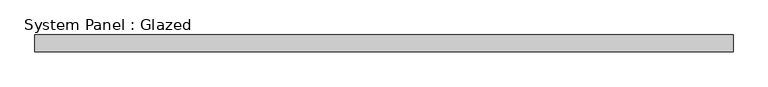
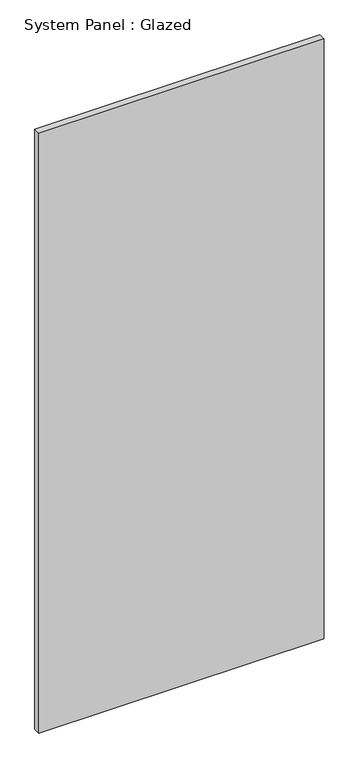
"""IFC4 building model written with IfcOpenShell, lengths in millimetres: plate geometry, System Panel : Glazed."""

from ifc_helpers import new_model, si_unit, origin, origin_with_axes, place, context, project, spatial, polyline, outline, extrude, source, transform, mapped, element, save


def system_panel_glazed_0266aec6(model_context):
    return source(origin(), model_context, "Body", "SweptSolid", [
        extrude(outline(polyline([(527.05, 19.05), (-527.05, 19.05), (-527.05, 44.45), (527.05, 44.45), (527.05, 19.05)])), origin_with_axes(), (0.0, 0.0, 1.0), 2343.15),
    ])


if __name__ == "__main__":
    model = new_model("IFC4")
    model_context = context("Model", 3, world=origin())
    ifc_project = project(units=[si_unit("LENGTHUNIT", "METRE", prefix="MILLI")], contexts=[model_context])
    site = spatial("IfcSite", under=ifc_project)
    building = spatial("IfcBuilding", under=site)
    placement = place(None, origin())
    system_panel_glazed_shape = system_panel_glazed_0266aec6(model_context)
    element("IfcPlate", 1, ObjectType="System Panel : Glazed", at=placement, inside=building, context=model_context, shape_type="MappedRepresentation", body=[
        mapped(system_panel_glazed_shape, transform((0.0, 0.0, 0.0), x_axis=(1.0, 0.0, 0.0), y_axis=(0.0, 1.0, 0.0), z_axis=(0.0, 0.0, 1.0))),
    ])
    save(model, "model.ifc")

# Revit data of these elements
# Type "System Panel : Glazed"
#   Construction Type Id = "GSP4R"
#   Analytic Construction = "1/8 in Pilkington single glazing"
#   Visual Light Transmittance = 0.9
#   Solar Heat Gain Coefficient = 0.86
#   Heat Transfer Coefficient (U) = 1.18115 BTU/(h·ft²·°F)
#   Define Thermal Properties by = 1
# Element 1 (IfcPlate, "System Panel : Glazed")
#   Materials on its faces: "Glass"
# Materials
#   "Glass": class "Glass", colour RGB 0 128 192, transparency 0.75, Description = "Soda Lime Glass", Cost = 0
